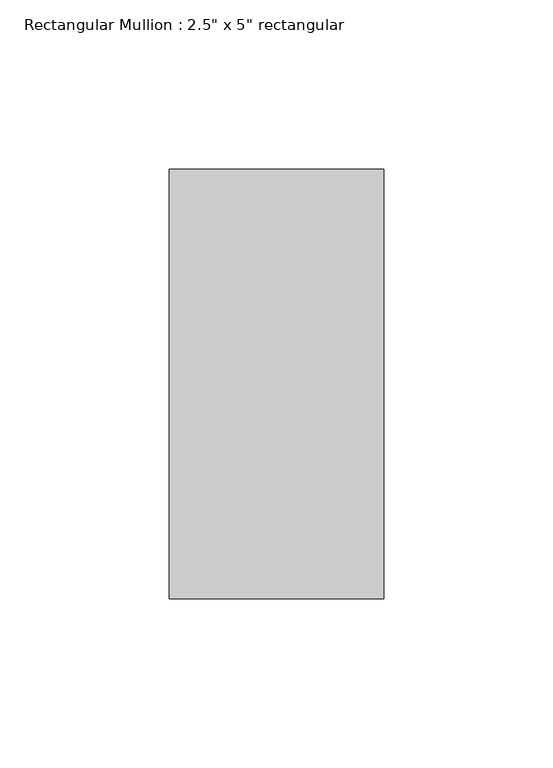
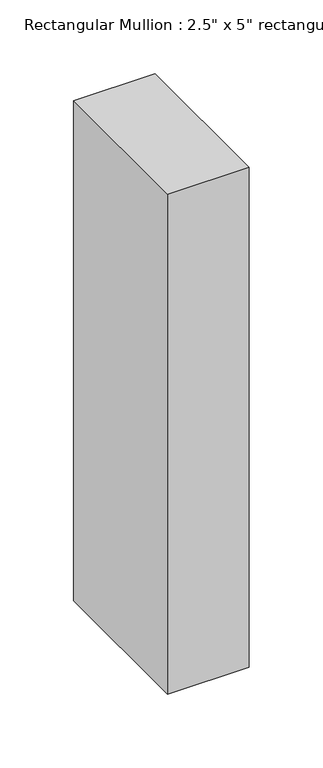
"""IFC4 building model written with IfcOpenShell, lengths in millimetres: member geometry."""

from ifc_helpers import new_model, si_unit, frame, origin, place, context, project, spatial, polyline, outline, extrude, source, transform, mapped, element, save


def member_5ae8a700(model_context):
    return source(origin(), model_context, "Body", "SweptSolid", [
        extrude(outline(polyline([(31.75, 63.5), (31.75, -63.5), (-31.75, -63.5), (-31.75, 63.5), (31.75, 63.5)])), frame((0.0, 0.0, -412.75), z_axis=(0.0, 0.0, 1.0), x_axis=(1.0, 0.0, 0.0)), (0.0, 0.0, 1.0), 412.75),
    ])


if __name__ == "__main__":
    model = new_model("IFC4")
    model_context = context("Model", 3, world=origin())
    ifc_project = project(units=[si_unit("LENGTHUNIT", "METRE", prefix="MILLI")], contexts=[model_context])
    site = spatial("IfcSite", under=ifc_project)
    building = spatial("IfcBuilding", under=site)
    placement = place(None, origin())
    member_shape = member_5ae8a700(model_context)
    element("IfcMember", 1, ObjectType="Rectangular Mullion : 2.5\" x 5\" rectangular", at=placement, inside=building, context=model_context, shape_type="MappedRepresentation", body=[
        mapped(member_shape, transform((0.0, 0.0, 0.0), x_axis=(1.0, 0.0, 0.0), y_axis=(0.0, 1.0, 0.0), z_axis=(0.0, 0.0, 1.0))),
    ])
    save(model, "model.ifc")

# Revit data of these elements
# Type "Rectangular Mullion : 2.5\" x 5\" rectangular"
#   built-in parameter 1007304 = 0.416667 (stored number, unit not read)
#   built-in parameter 1007301 = 0.104167 (stored number, unit not read)
#   built-in parameter 1007300 = 0.104167 (stored number, unit not read)
